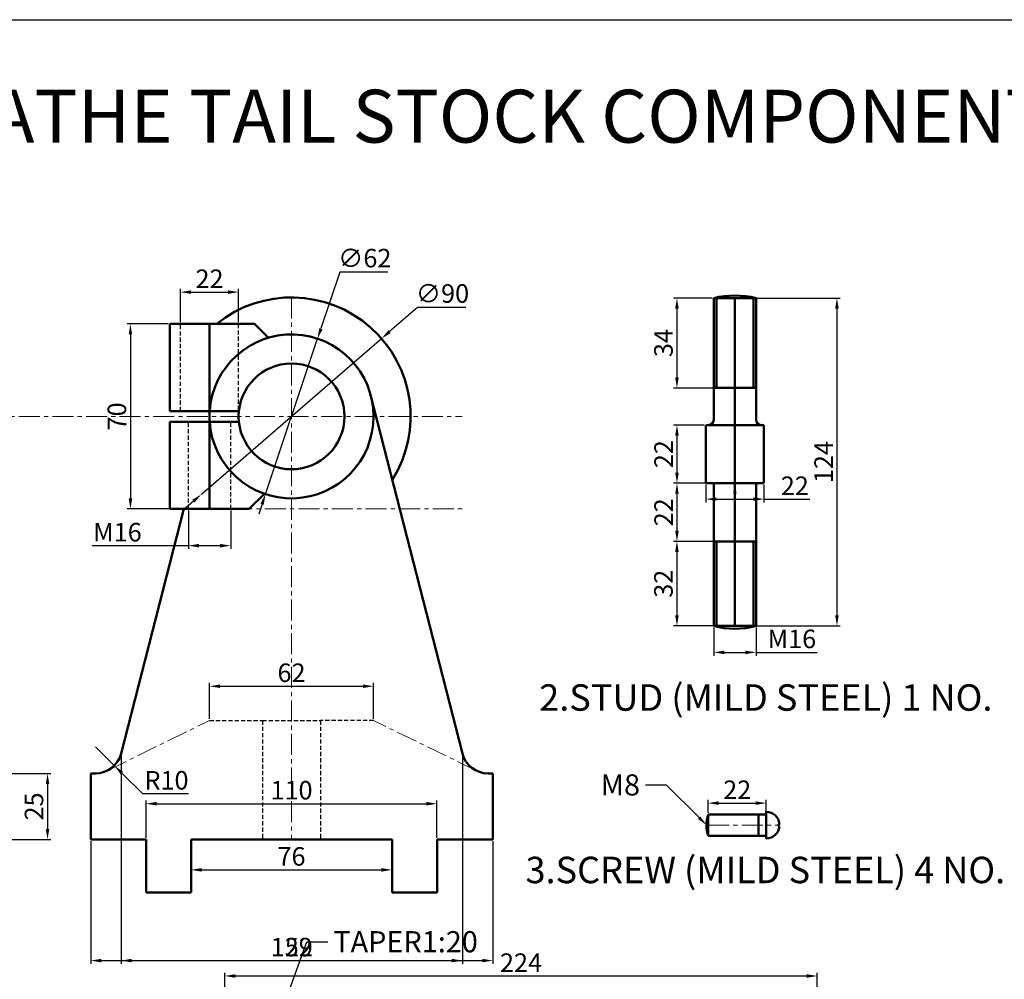
# Model space of a CAD drawing. Units: millimetres. Extents: x -66 to 1195, y -396 to 398.
# Tile 5 of 8: x 373 to 745, y 35 to 398. Entities that reach past the tile are written whole.
import ezdxf
from ezdxf import colors
from ezdxf.entities.mleader import LeaderData, LeaderLine
from ezdxf.math import Vec2, Vec3

# ---------------------------------------------------------------- set-up
doc = ezdxf.new("R2010")
doc.units = ezdxf.units.MM
doc.header["$LTSCALE"] = 0.5
doc.linetypes.add('CENTER', pattern=[50.8, 31.75, -6.35, 6.35, -6.35])
doc.linetypes.add('HIDDEN', pattern=[9.525, 6.35, -3.175])
for name, color, linetype, lineweight in [('M-CNTR', 1, 'CENTER', 18), ('M-DIMS', 2, 'Continuous', 25), ('M-HIDN', 3, 'HIDDEN', 25), ('M-OUTL', 7, 'Continuous', 50), ('M-TEXT', 7, 'Continuous', 25), ('M-TTLB', 7, 'Continuous', 25)]:
    doc.layers.add(name, color=color, linetype=linetype, lineweight=lineweight)
doc.styles.get("Standard").update_dxf_attribs({"font": 'arial.ttf'})
doc.dimstyles.new('ISO-25', dxfattribs={"dimtxt": 7, "dimasz": 4, "dimexe": 1.25, "dimexo": 0.625, "dimtad": 1, "dimtoh": 1, "dimtxsty": 'Standard', "dimcen": 2.5, "dimadec": 0, "dimazin": 0, "dimtfac": 1, "dimtmove": 0, "dimatfit": 3, "dimfxl": 1, "dimarcsym": 0})

# ---------------------------------------------------------------- blocks, each defined once
blk = doc.blocks.new('*D30')
at = {"layer": 'Defpoints', "color": 0, "ltscale": 0.5, "transparency": 16777216}
for p in [(185.07, 112.61), (185.07, 87.61), (383.19, 87.61)]:
    blk.add_point(p, dxfattribs=at)
at = {"layer": 'M-DIMS', "color": 0, "lineweight": -2, "ltscale": 0.5, "transparency": 16777216}
for p, q in [((185.69, 112.61), (384.44, 112.61)), ((383.19, 108.61), (383.19, 91.61)), ((185.69, 87.61), (384.44, 87.61))]:
    blk.add_line(p, q, dxfattribs=at)
at = {"layer": 'M-DIMS', "color": 0, "ltscale": 0.5, "transparency": 16777216}
for points in [[(382.52, 108.61), (383.85, 108.61), (383.19, 112.61)], [(382.52, 91.61), (383.85, 91.61), (383.19, 87.61)]]:
    blk.add_solid(points, dxfattribs=at)
at = {"layer": 'M-DIMS', "color": 0, "ltscale": 0.5, "transparency": 16777216, "insert": (378.99, 100.11), "char_height": 7, "attachment_point": 5, "rotation": 90}
blk.add_mtext('25', dxfattribs=at)
blk = doc.blocks.new('*D31')
at = {"layer": 'Defpoints', "color": 0, "ltscale": 0.5, "transparency": 16777216}
for p in [(506.43, 145.56), (444.43, 132.61), (506.43, 132.61)]:
    blk.add_point(p, dxfattribs=at)
at = {"layer": 'M-DIMS', "color": 0, "lineweight": -2, "ltscale": 0.5, "transparency": 16777216}
for p, q in [((444.43, 133.24), (444.43, 146.81)), ((448.43, 145.56), (502.43, 145.56)), ((506.43, 133.24), (506.43, 146.81))]:
    blk.add_line(p, q, dxfattribs=at)
at = {"layer": 'M-DIMS', "color": 0, "ltscale": 0.5, "transparency": 16777216}
for points in [[(448.43, 146.22), (448.43, 144.89), (444.43, 145.56)], [(502.43, 146.22), (502.43, 144.89), (506.43, 145.56)]]:
    blk.add_solid(points, dxfattribs=at)
at = {"layer": 'M-DIMS', "color": 0, "ltscale": 0.5, "transparency": 16777216, "insert": (475.43, 149.76), "char_height": 7, "attachment_point": 5}
blk.add_mtext('62', dxfattribs=at)
blk = doc.blocks.new('*D32')
at = {"layer": 'Defpoints', "color": 0, "ltscale": 0.5, "transparency": 16777216}
for p in [(530.43, 101.14), (420.43, 87.61), (530.43, 87.61)]:
    blk.add_point(p, dxfattribs=at)
at = {"layer": 'M-DIMS', "color": 0, "lineweight": -2, "ltscale": 0.5, "transparency": 16777216}
for p, q in [((420.43, 88.24), (420.43, 102.39)), ((424.43, 101.14), (526.43, 101.14)), ((530.43, 88.24), (530.43, 102.39))]:
    blk.add_line(p, q, dxfattribs=at)
at = {"layer": 'M-DIMS', "color": 0, "ltscale": 0.5, "transparency": 16777216}
for points in [[(424.43, 101.81), (424.43, 100.48), (420.43, 101.14)], [(526.43, 101.81), (526.43, 100.48), (530.43, 101.14)]]:
    blk.add_solid(points, dxfattribs=at)
at = {"layer": 'M-DIMS', "color": 0, "ltscale": 0.5, "transparency": 16777216, "insert": (475.43, 105.34), "char_height": 7, "attachment_point": 5}
blk.add_mtext('110', dxfattribs=at)
blk = doc.blocks.new('*D33')
at = {"layer": 'Defpoints', "color": 0, "ltscale": 0.5, "transparency": 16777216}
for p in [(437.43, 87.61), (513.43, 87.61), (513.43, 76.11)]:
    blk.add_point(p, dxfattribs=at)
at = {"layer": 'M-DIMS', "color": 0, "lineweight": -2, "ltscale": 0.5, "transparency": 16777216}
for p, q in [((437.43, 86.99), (437.43, 74.86)), ((513.43, 86.99), (513.43, 74.86)), ((441.43, 76.11), (509.43, 76.11))]:
    blk.add_line(p, q, dxfattribs=at)
at = {"layer": 'M-DIMS', "color": 0, "ltscale": 0.5, "transparency": 16777216}
for points in [[(441.43, 76.78), (441.43, 75.44), (437.43, 76.11)], [(509.43, 76.78), (509.43, 75.44), (513.43, 76.11)]]:
    blk.add_solid(points, dxfattribs=at)
at = {"layer": 'M-DIMS', "color": 0, "ltscale": 0.5, "transparency": 16777216, "insert": (475.43, 80.31), "char_height": 7, "attachment_point": 5}
blk.add_mtext('76', dxfattribs=at)
blk = doc.blocks.new('*D34')
at = {"layer": 'Defpoints', "color": 0, "ltscale": 0.5, "transparency": 16777216}
for p in [(429.43, 282.61), (414.53, 212.61), (429.43, 212.61)]:
    blk.add_point(p, dxfattribs=at)
at = {"layer": 'M-DIMS', "color": 0, "lineweight": -2, "ltscale": 0.5, "transparency": 16777216}
for p, q in [((428.81, 282.61), (413.28, 282.61)), ((414.53, 278.61), (414.53, 216.61)), ((428.81, 212.61), (413.28, 212.61))]:
    blk.add_line(p, q, dxfattribs=at)
at = {"layer": 'M-DIMS', "color": 0, "ltscale": 0.5, "transparency": 16777216}
for points in [[(413.87, 278.61), (415.2, 278.61), (414.53, 282.61)], [(413.87, 216.61), (415.2, 216.61), (414.53, 212.61)]]:
    blk.add_solid(points, dxfattribs=at)
at = {"layer": 'M-DIMS', "color": 0, "ltscale": 0.5, "transparency": 16777216, "insert": (410.33, 247.61), "char_height": 7, "attachment_point": 5, "rotation": 90}
blk.add_mtext('70', dxfattribs=at)
blk = doc.blocks.new('*D35')
at = {"layer": 'Defpoints', "color": 0, "ltscale": 0.5, "transparency": 16777216}
for p in [(455.43, 294.62), (433.43, 282.61), (455.43, 282.61)]:
    blk.add_point(p, dxfattribs=at)
at = {"layer": 'M-DIMS', "color": 0, "lineweight": -2, "ltscale": 0.5, "transparency": 16777216}
for p, q in [((433.43, 283.24), (433.43, 295.87)), ((437.43, 294.62), (451.43, 294.62)), ((455.43, 283.24), (455.43, 295.87))]:
    blk.add_line(p, q, dxfattribs=at)
at = {"layer": 'M-DIMS', "color": 0, "ltscale": 0.5, "transparency": 16777216}
for points in [[(437.43, 295.29), (437.43, 293.95), (433.43, 294.62)], [(451.43, 295.29), (451.43, 293.95), (455.43, 294.62)]]:
    blk.add_solid(points, dxfattribs=at)
at = {"layer": 'M-DIMS', "color": 0, "ltscale": 0.5, "transparency": 16777216, "insert": (444.43, 298.76), "char_height": 7, "attachment_point": 5}
blk.add_mtext('22', dxfattribs=at)
blk = doc.blocks.new('*D36')
at = {"layer": 'Defpoints', "color": 0, "ltscale": 0.5, "transparency": 16777216}
for p in [(436.43, 212.61), (452.43, 212.61), (452.43, 198.72)]:
    blk.add_point(p, dxfattribs=at)
at = {"layer": 'M-DIMS', "color": 0, "lineweight": -2, "ltscale": 0.5, "transparency": 16777216}
for p, q in [((436.43, 211.99), (436.43, 197.47)), ((452.43, 211.99), (452.43, 197.47)), ((436.43, 198.72), (400.07, 198.72)), ((448.43, 198.72), (440.43, 198.72))]:
    blk.add_line(p, q, dxfattribs=at)
at = {"layer": 'M-DIMS', "color": 0, "ltscale": 0.5, "transparency": 16777216}
for points in [[(440.43, 199.39), (440.43, 198.06), (436.43, 198.72)], [(448.43, 199.39), (448.43, 198.06), (452.43, 198.72)]]:
    blk.add_solid(points, dxfattribs=at)
at = {"layer": 'M-DIMS', "color": 0, "ltscale": 0.5, "transparency": 16777216, "insert": (409.62, 202.92), "char_height": 7, "attachment_point": 5}
blk.add_mtext('M16', dxfattribs=at)
blk = doc.blocks.new('*D37')
at = {"layer": 'Defpoints', "color": 0, "ltscale": 0.5, "transparency": 16777216}
for p in [(509.47, 277.04), (441.39, 218.18)]:
    blk.add_point(p, dxfattribs=at)
at = {"layer": 'M-DIMS', "color": 0, "lineweight": -2, "ltscale": 0.5, "transparency": 16777216}
for p, q in [((523.06, 288.79), (512.5, 279.66)), ((541.31, 288.79), (523.06, 288.79)), ((441.39, 218.18), (509.47, 277.04)), ((438.37, 215.56), (435.34, 212.95))]:
    blk.add_line(p, q, dxfattribs=at)
at = {"layer": 'M-DIMS', "color": 0, "ltscale": 0.5, "transparency": 16777216}
for points in [[(512.06, 280.16), (512.94, 279.15), (509.47, 277.04)], [(437.93, 216.07), (438.8, 215.06), (441.39, 218.18)]]:
    blk.add_solid(points, dxfattribs=at)
at = {"layer": 'M-DIMS', "color": 0, "ltscale": 0.5, "transparency": 16777216, "insert": (532.5, 293.19), "char_height": 7, "attachment_point": 5}
blk.add_mtext('∅90', dxfattribs=at)
blk = doc.blocks.new('*D38')
at = {"layer": 'Defpoints', "color": 0, "ltscale": 0.5, "transparency": 16777216}
for p in [(485.28, 277.01), (465.59, 218.22)]:
    blk.add_point(p, dxfattribs=at)
at = {"layer": 'M-DIMS', "color": 0, "lineweight": -2, "ltscale": 0.5, "transparency": 16777216}
for p, q in [((493.7, 302.17), (486.55, 280.8)), ((511.9, 302.17), (493.7, 302.17)), ((465.59, 218.22), (485.28, 277.01)), ((464.32, 214.42), (463.05, 210.63))]:
    blk.add_line(p, q, dxfattribs=at)
at = {"layer": 'M-DIMS', "color": 0, "ltscale": 0.5, "transparency": 16777216}
for points in [[(485.91, 281.01), (487.18, 280.59), (485.28, 277.01)], [(463.69, 214.63), (464.95, 214.21), (465.59, 218.22)]]:
    blk.add_solid(points, dxfattribs=at)
at = {"layer": 'M-DIMS', "color": 0, "ltscale": 0.5, "transparency": 16777216, "insert": (503.12, 306.57), "char_height": 7, "attachment_point": 5}
blk.add_mtext('∅62', dxfattribs=at)
blk = doc.blocks.new('*D39')
at = {"layer": 'Defpoints', "color": 0, "ltscale": 0.5, "transparency": 16777216}
for p in [(635.05, 292.35), (621.15, 258.35), (636.05, 258.35)]:
    blk.add_point(p, dxfattribs=at)
at = {"layer": 'M-DIMS', "color": 0, "lineweight": -2, "ltscale": 0.5, "transparency": 16777216}
for p, q in [((634.42, 292.35), (619.9, 292.35)), ((621.15, 288.35), (621.15, 262.35)), ((635.42, 258.35), (619.9, 258.35))]:
    blk.add_line(p, q, dxfattribs=at)
at = {"layer": 'M-DIMS', "color": 0, "ltscale": 0.5, "transparency": 16777216}
for points in [[(620.48, 288.35), (621.81, 288.35), (621.15, 292.35)], [(620.48, 262.35), (621.81, 262.35), (621.15, 258.35)]]:
    blk.add_solid(points, dxfattribs=at)
at = {"layer": 'M-DIMS', "color": 0, "ltscale": 0.5, "transparency": 16777216, "insert": (616.95, 275.35), "char_height": 7, "attachment_point": 5, "rotation": 90}
blk.add_mtext('34', dxfattribs=at)
blk = doc.blocks.new('*D40')
at = {"layer": 'Defpoints', "color": 0, "ltscale": 0.5, "transparency": 16777216}
for p in [(632.05, 222.35), (654.05, 222.35), (654.05, 216.33)]:
    blk.add_point(p, dxfattribs=at)
at = {"layer": 'M-DIMS', "color": 0, "lineweight": -2, "ltscale": 0.5, "transparency": 16777216}
for p, q in [((632.05, 221.73), (632.05, 215.08)), ((654.05, 221.73), (654.05, 215.08)), ((636.05, 216.33), (650.05, 216.33)), ((654.05, 216.33), (671.37, 216.33))]:
    blk.add_line(p, q, dxfattribs=at)
at = {"layer": 'M-DIMS', "color": 0, "ltscale": 0.5, "transparency": 16777216}
for points in [[(636.05, 216.99), (636.05, 215.66), (632.05, 216.33)], [(650.05, 216.99), (650.05, 215.66), (654.05, 216.33)]]:
    blk.add_solid(points, dxfattribs=at)
at = {"layer": 'M-DIMS', "color": 0, "ltscale": 0.5, "transparency": 16777216, "insert": (665.71, 220.47), "char_height": 7, "attachment_point": 5}
blk.add_mtext('22', dxfattribs=at)
blk = doc.blocks.new('*D41')
at = {"layer": 'Defpoints', "color": 0, "ltscale": 0.5, "transparency": 16777216}
for p in [(632.05, 244.35), (621.15, 222.35), (632.05, 222.35)]:
    blk.add_point(p, dxfattribs=at)
at = {"layer": 'M-DIMS', "color": 0, "lineweight": -2, "ltscale": 0.5, "transparency": 16777216}
for p, q in [((631.42, 244.35), (619.9, 244.35)), ((621.15, 240.35), (621.15, 226.35)), ((631.42, 222.35), (619.9, 222.35))]:
    blk.add_line(p, q, dxfattribs=at)
at = {"layer": 'M-DIMS', "color": 0, "ltscale": 0.5, "transparency": 16777216}
for points in [[(620.48, 240.35), (621.81, 240.35), (621.15, 244.35)], [(620.48, 226.35), (621.81, 226.35), (621.15, 222.35)]]:
    blk.add_solid(points, dxfattribs=at)
at = {"layer": 'M-DIMS', "color": 0, "ltscale": 0.5, "transparency": 16777216, "insert": (617.01, 233.35), "char_height": 7, "attachment_point": 5, "rotation": 90}
blk.add_mtext('22', dxfattribs=at)
blk = doc.blocks.new('*D42')
at = {"layer": 'Defpoints', "color": 0, "ltscale": 0.5, "transparency": 16777216}
for p in [(643.05, 222.35), (621.15, 200.35), (643.05, 200.35)]:
    blk.add_point(p, dxfattribs=at)
at = {"layer": 'M-DIMS', "color": 0, "lineweight": -2, "ltscale": 0.5, "transparency": 16777216}
for p, q in [((642.42, 222.35), (619.9, 222.35)), ((621.15, 218.35), (621.15, 204.35)), ((642.42, 200.35), (619.9, 200.35))]:
    blk.add_line(p, q, dxfattribs=at)
at = {"layer": 'M-DIMS', "color": 0, "ltscale": 0.5, "transparency": 16777216}
for points in [[(620.48, 218.35), (621.81, 218.35), (621.15, 222.35)], [(620.48, 204.35), (621.81, 204.35), (621.15, 200.35)]]:
    blk.add_solid(points, dxfattribs=at)
at = {"layer": 'M-DIMS', "color": 0, "ltscale": 0.5, "transparency": 16777216, "insert": (617.01, 211.35), "char_height": 7, "attachment_point": 5, "rotation": 90}
blk.add_mtext('22', dxfattribs=at)
blk = doc.blocks.new('*D43')
at = {"layer": 'Defpoints', "color": 0, "ltscale": 0.5, "transparency": 16777216}
for p in [(643.05, 200.35), (621.15, 168.35), (643.05, 168.35)]:
    blk.add_point(p, dxfattribs=at)
at = {"layer": 'M-DIMS', "color": 0, "lineweight": -2, "ltscale": 0.5, "transparency": 16777216}
for p, q in [((642.42, 200.35), (619.9, 200.35)), ((621.15, 196.35), (621.15, 172.35)), ((642.42, 168.35), (619.9, 168.35))]:
    blk.add_line(p, q, dxfattribs=at)
at = {"layer": 'M-DIMS', "color": 0, "ltscale": 0.5, "transparency": 16777216}
for points in [[(620.48, 196.35), (621.81, 196.35), (621.15, 200.35)], [(620.48, 172.35), (621.81, 172.35), (621.15, 168.35)]]:
    blk.add_solid(points, dxfattribs=at)
at = {"layer": 'M-DIMS', "color": 0, "ltscale": 0.5, "transparency": 16777216, "insert": (616.95, 184.35), "char_height": 7, "attachment_point": 5, "rotation": 90}
blk.add_mtext('32', dxfattribs=at)
blk = doc.blocks.new('*D44')
at = {"layer": 'Defpoints', "color": 0, "ltscale": 0.5, "transparency": 16777216}
for p in [(635.05, 168.35), (651.05, 168.35), (651.05, 158.37)]:
    blk.add_point(p, dxfattribs=at)
at = {"layer": 'M-DIMS', "color": 0, "lineweight": -2, "ltscale": 0.5, "transparency": 16777216}
for p, q in [((635.05, 167.73), (635.05, 157.12)), ((651.05, 167.73), (651.05, 157.12)), ((639.05, 158.37), (647.05, 158.37)), ((651.05, 158.37), (674.15, 158.37))]:
    blk.add_line(p, q, dxfattribs=at)
at = {"layer": 'M-DIMS', "color": 0, "ltscale": 0.5, "transparency": 16777216}
for points in [[(639.05, 159.04), (639.05, 157.7), (635.05, 158.37)], [(647.05, 159.04), (647.05, 157.7), (651.05, 158.37)]]:
    blk.add_solid(points, dxfattribs=at)
at = {"layer": 'M-DIMS', "color": 0, "ltscale": 0.5, "transparency": 16777216, "insert": (664.6, 162.57), "char_height": 7, "attachment_point": 5}
blk.add_mtext('M16', dxfattribs=at)
blk = doc.blocks.new('*D45')
at = {"layer": 'Defpoints', "color": 0, "ltscale": 0.5, "transparency": 16777216}
for p in [(643.05, 292.35), (643.05, 168.35), (681.63, 168.35)]:
    blk.add_point(p, dxfattribs=at)
at = {"layer": 'M-DIMS', "color": 0, "lineweight": -2, "ltscale": 0.5, "transparency": 16777216}
for p, q in [((643.67, 292.35), (682.88, 292.35)), ((681.63, 288.35), (681.63, 172.35)), ((643.67, 168.35), (682.88, 168.35))]:
    blk.add_line(p, q, dxfattribs=at)
at = {"layer": 'M-DIMS', "color": 0, "ltscale": 0.5, "transparency": 16777216}
for points in [[(680.97, 288.35), (682.3, 288.35), (681.63, 292.35)], [(680.97, 172.35), (682.3, 172.35), (681.63, 168.35)]]:
    blk.add_solid(points, dxfattribs=at)
at = {"layer": 'M-DIMS', "color": 0, "ltscale": 0.5, "transparency": 16777216, "insert": (677.49, 230.35), "char_height": 7, "attachment_point": 5, "rotation": 90}
blk.add_mtext('124', dxfattribs=at)
blk = doc.blocks.new('*D46')
at = {"layer": 'Defpoints', "color": 0, "ltscale": 0.5, "transparency": 16777216}
for p in [(654.93, 101.37), (632.93, 97.04), (654.93, 97.54)]:
    blk.add_point(p, dxfattribs=at)
at = {"layer": 'M-DIMS', "color": 0, "lineweight": -2, "ltscale": 0.5, "transparency": 16777216}
for p, q in [((632.93, 97.67), (632.93, 102.62)), ((636.93, 101.37), (650.93, 101.37)), ((654.93, 98.17), (654.93, 102.62))]:
    blk.add_line(p, q, dxfattribs=at)
at = {"layer": 'M-DIMS', "color": 0, "ltscale": 0.5, "transparency": 16777216}
for points in [[(636.93, 102.04), (636.93, 100.7), (632.93, 101.37)], [(650.93, 102.04), (650.93, 100.7), (654.93, 101.37)]]:
    blk.add_solid(points, dxfattribs=at)
at = {"layer": 'M-DIMS', "color": 0, "ltscale": 0.5, "transparency": 16777216, "insert": (643.93, 105.51), "char_height": 7, "attachment_point": 5}
blk.add_mtext('22', dxfattribs=at)
blk = doc.blocks.new('*D50')
at = {"layer": 'Defpoints', "color": 0, "ltscale": 0.5, "transparency": 16777216}
for p in [(674.2, 35.99), (450.2, 28.9), (674.2, 28.9)]:
    blk.add_point(p, dxfattribs=at)
at = {"layer": 'M-DIMS', "color": 0, "lineweight": -2, "ltscale": 0.5, "transparency": 16777216}
for p, q in [((450.2, 29.53), (450.2, 37.24)), ((674.2, 29.53), (674.2, 37.24)), ((454.2, 35.99), (670.2, 35.99))]:
    blk.add_line(p, q, dxfattribs=at)
at = {"layer": 'M-DIMS', "color": 0, "ltscale": 0.5, "transparency": 16777216}
for points in [[(454.2, 36.65), (454.2, 35.32), (450.2, 35.99)], [(670.2, 36.65), (670.2, 35.32), (674.2, 35.99)]]:
    blk.add_solid(points, dxfattribs=at)
at = {"layer": 'M-DIMS', "color": 0, "ltscale": 0.5, "transparency": 16777216, "insert": (562.2, 40.13), "char_height": 7, "attachment_point": 5}
blk.add_mtext('224', dxfattribs=at)
blk = doc.blocks.new('*D103')
at = {"layer": 'Defpoints', "color": 0, "ltscale": 0.5, "transparency": 16777216}
for p in [(399.53, 87.61), (551.53, 87.61), (551.53, 41.81)]:
    blk.add_point(p, dxfattribs=at)
at = {"layer": 'M-DIMS', "color": 0, "lineweight": -2, "ltscale": 0.5, "transparency": 16777216}
for p, q in [((399.53, 86.99), (399.53, 40.56)), ((551.53, 86.99), (551.53, 40.56)), ((403.53, 41.81), (547.53, 41.81))]:
    blk.add_line(p, q, dxfattribs=at)
at = {"layer": 'M-DIMS', "color": 0, "ltscale": 0.5, "transparency": 16777216}
for points in [[(403.53, 42.48), (403.53, 41.14), (399.53, 41.81)], [(547.53, 42.48), (547.53, 41.14), (551.53, 41.81)]]:
    blk.add_solid(points, dxfattribs=at)
at = {"layer": 'M-DIMS', "color": 0, "ltscale": 0.5, "transparency": 16777216, "insert": (475.53, 46.01), "char_height": 7, "attachment_point": 5}
blk.add_mtext('152', dxfattribs=at)
blk = doc.blocks.new('*D104')
at = {"layer": 'Defpoints', "color": 0, "ltscale": 0.5, "transparency": 16777216}
for p in [(411.03, 120.13), (540.03, 120.13), (540.03, 41.81)]:
    blk.add_point(p, dxfattribs=at)
at = {"layer": 'M-DIMS', "color": 0, "lineweight": -2, "ltscale": 0.5, "transparency": 16777216}
for p, q in [((411.03, 119.51), (411.03, 40.56)), ((540.03, 119.51), (540.03, 40.56)), ((415.03, 41.81), (536.03, 41.81))]:
    blk.add_line(p, q, dxfattribs=at)
at = {"layer": 'M-DIMS', "color": 0, "ltscale": 0.5, "transparency": 16777216}
for points in [[(415.03, 42.48), (415.03, 41.14), (411.03, 41.81)], [(536.03, 42.48), (536.03, 41.14), (540.03, 41.81)]]:
    blk.add_solid(points, dxfattribs=at)
at = {"layer": 'M-DIMS', "color": 0, "ltscale": 0.5, "transparency": 16777216, "insert": (475.53, 46.01), "char_height": 7, "attachment_point": 5}
blk.add_mtext('129', dxfattribs=at)
blk = doc.blocks.new('*D118')
at = {"layer": 'Defpoints', "color": 0, "ltscale": 0.5, "transparency": 16777216}
for p in [(401.34, 122.61), (408.44, 115.56)]:
    blk.add_point(p, dxfattribs=at)
at = {"layer": 'M-DIMS', "color": 0, "lineweight": -2, "ltscale": 0.5, "transparency": 16777216}
for p, q in [((401.34, 122.61), (408.44, 115.56)), ((419.18, 104.89), (411.27, 112.74)), ((436.51, 104.89), (419.18, 104.89))]:
    blk.add_line(p, q, dxfattribs=at)
at = {"layer": 'M-DIMS', "color": 0, "ltscale": 0.5, "transparency": 16777216}
blk.add_solid([(411.74, 113.22), (410.8, 112.27), (408.44, 115.56)], dxfattribs=at)
at = {"layer": 'M-DIMS', "color": 0, "ltscale": 0.5, "transparency": 16777216, "insert": (428.16, 109.09), "char_height": 7, "attachment_point": 5}
blk.add_mtext('R10', dxfattribs=at)

msp = doc.modelspace()

# ---------------------------------------------------------------- linework, layer by layer
at = {"layer": 'M-CNTR', "ltscale": 0.5}
for p, q in [((475.4327, 292.6106), (475.4327, 87.6106)), ((346.9367, 247.6106), (539.9794, 247.6106)), ((414.5332, 212.6106), (539.9794, 212.6106)), ((405.7453, 113.6326), (444.4327, 132.6106)), ((545.3342, 113.6238), (506.4327, 132.6106)), ((632.9262, 93.0426), (659.3995, 93.0426))]:
    msp.add_line(p, q, dxfattribs=at)
at = {"layer": 'M-HIDN', "ltscale": 0.5}
for p, q in [((433.4327, 249.6106), (433.4327, 282.6106)), ((455.4327, 247.6106), (455.4327, 282.6106)), ((436.4327, 212.6106), (436.4327, 245.6106)), ((452.4327, 212.6106), (452.4327, 245.6106)), ((444.4327, 132.6106), (464.4327, 132.6106)), ((464.4327, 132.6106), (486.4327, 132.6106)), ((464.4327, 132.6106), (464.4327, 87.6106)), ((486.4327, 132.6106), (486.4327, 87.6106)), ((506.4327, 132.6106), (486.4327, 132.6106))]:
    msp.add_line(p, q, dxfattribs=at)
at = {"layer": 'M-OUTL', "ltscale": 0.5}
for p, q in [((635.0478, 292.3534), (651.0478, 292.3534)), ((635.0478, 246.3534), (635.0478, 292.3534)), ((636.0478, 258.3534), (636.0478, 292.3534)), ((643.0478, 292.3534), (643.0478, 168.3534)), ((650.0478, 292.3534), (650.0478, 258.3534)), ((651.0478, 292.3534), (651.0478, 246.3534)), ((429.4327, 249.6106), (429.4327, 282.6106)), ((429.4327, 282.6106), (461.4327, 282.6106)), ((444.4327, 249.6106), (444.4327, 282.6106)), ((461.4327, 282.6106), (466.6908, 277.3525)), ((651.0478, 258.3534), (635.0478, 258.3534)), ((643.0478, 258.3534), (643.0478, 242.3534)), ((505.4661, 255.2915), (540.0322, 120.1329)), ((429.4327, 249.6106), (455.533, 249.6106)), ((444.4327, 212.6106), (444.4327, 249.6106)), ((429.4327, 212.6106), (429.4327, 245.6106)), ((429.4327, 245.6106), (455.533, 245.6106)), ((632.0478, 244.3534), (632.0478, 222.3534)), ((633.0478, 244.3534), (632.0478, 244.3534)), ((654.0478, 244.3534), (633.0478, 244.3534)), ((654.0478, 244.3534), (654.0478, 222.3534)), ((632.0478, 222.3534), (654.0478, 222.3534)), ((635.0478, 222.3534), (635.0478, 168.3534)), ((643.0478, 222.3534), (643.0478, 200.3534)), ((643.0478, 222.3534), (643.0478, 200.3534)), ((651.0478, 222.3534), (651.0478, 168.3534)), ((459.4327, 212.6106), (465.178, 218.3558)), ((434.6801, 212.6106), (411.0294, 120.1329)), ((429.4327, 212.6106), (459.4327, 212.6106)), ((635.0478, 200.3534), (651.0478, 200.3534)), ((636.0478, 200.3534), (636.0478, 168.3534)), ((650.0478, 200.3534), (650.0478, 168.3534)), ((635.0478, 168.3534), (651.0478, 168.3534)), ((399.5308, 112.6106), (401.3412, 112.6106)), ((399.5308, 112.6106), (399.5308, 87.6106)), ((549.7204, 112.6106), (551.5308, 112.6106)), ((551.5308, 112.6106), (551.5308, 87.6106)), ((632.9262, 97.0426), (654.9262, 97.0426)), ((632.9262, 89.0426), (632.9262, 97.0426)), ((651.9262, 97.0426), (651.9262, 89.0426)), ((654.9262, 97.0426), (654.9262, 98.0426)), ((654.9262, 97.0426), (654.9262, 89.0426)), ((659.901, 93.5441), (659.3995, 93.0426)), ((659.901, 92.541), (659.3995, 93.0426)), ((399.5308, 87.6106), (420.4327, 87.6106)), ((420.4327, 87.6106), (420.4327, 67.6106)), ((437.4327, 87.6106), (437.4327, 67.6106)), ((437.4327, 87.6106), (513.4327, 87.6106)), ((513.4327, 87.6106), (513.4327, 67.6106)), ((530.4327, 87.6106), (530.4327, 67.6106)), ((530.4327, 87.6106), (551.5308, 87.6106)), ((654.9262, 89.0426), (632.9262, 89.0426)), ((654.9262, 89.0426), (654.9262, 88.0426)), ((420.4327, 67.6106), (437.4327, 67.6106)), ((513.4327, 67.6106), (530.4327, 67.6106))]:
    msp.add_line(p, q, dxfattribs=at)
msp.add_circle((475.4327, 247.6106), 20, dxfattribs=at)
for centre, radius, start, end in [((475.4327, 247.6106), 45, 327.887824, 128.942441), ((643.0478, 259.7431), 33.5772, 76.21633, 103.78367), ((475.4327, 247.6106), 31, 183.699071, 176.300929), ((633.0478, 246.3534), 2, 270, 0), ((653.0478, 246.3534), 2, 180, 270), ((643.0478, 198.7001), 31.3835, 255.231697, 284.768303), ((401.3412, 122.6106), 10, 270, 345.654395), ((549.7204, 122.6106), 10, 194.345605, 270), ((646.2508, 93.0426), 13.9121, 163.290472, 196.709528), ((654.9262, 93.0426), 5, 5.75663, 90), ((654.9262, 93.0426), 5, 270, 354.24337)]:
    msp.add_arc(centre, radius, start, end, dxfattribs=at)
at = {"layer": 'M-TTLB', "ltscale": 0.5}
msp.add_lwpolyline([(-66.4176, 397.641), (1195.0519, 397.641), (1195.0519, -395.6964), (-66.4176, -395.6964)], close=True, dxfattribs=at)

# ---------------------------------------------------------------- texts
at = {"layer": 'M-TEXT', "ltscale": 0.5, "attachment_point": 1}
for s, width, insert, char_height in [('LATHE TAIL STOCK COMPONENTS ', 485.790741, (346.8576, 371.1482), 20), ('\\pxqc;2.STUD (MILD STEEL) 1 NO.', 191.333714, (559.0807, 146.3007), 10), ('\\pxqc;3.SCREW (MILD STEEL) 4 NO.', 203.992441, (552.5644, 81.0812), 10)]:
    msp.add_mtext_dynamic_manual_height_columns(s, width=width, gutter_width=12.5, heights=[0], dxfattribs=dict(at, insert=insert, char_height=char_height))

# ---------------------------------------------------------------- dimensions: what is measured, and where the dimension line sits
at = {"layer": 'M-DIMS', "ltscale": 0.5}
for p1, p2, picture, middle in [((465.5888, 218.215), (485.2766, 277.0061), '*D38', (503.1153, 302.1731)), ((441.3921, 218.1787), (509.4733, 277.0425), '*D37', (532.4958, 288.7907))]:
    dim = msp.add_diameter_dim_2p(p1=p1, p2=p2, dimstyle='ISO-25', override={"dimclrd": 0, "dimclre": 0, "dimclrt": 0}, dxfattribs=at)
    dim.commit()
    dim.dimension.update_dxf_attribs({"geometry": picture, "text_midpoint": middle, "dimtype": 163})
for base, p1, p2, override, picture, middle in [((455.4327, 294.621), (433.4327, 282.6106), (455.4327, 282.6106), {"dimclrd": 0, "dimclre": 0, "dimclrt": 0}, '*D35', (444.4327, 298.7604)), ((506.4327, 145.5566), (444.4327, 132.6106), (506.4327, 132.6106), {"dimclrd": 0, "dimclre": 0, "dimclrt": 0}, '*D31', (475.4327, 149.7556)), ((540.0322, 41.8106), (411.0294, 120.1329), (540.0322, 120.1329), {"dimdec": 0, "dimlfac": 1, "dimrnd": 0, "dimzin": 0, "dimdsep": 46, "dimlunit": 2}, '*D104', (475.5308, 46.0096)), ((530.4327, 101.1427), (420.4327, 87.6106), (530.4327, 87.6106), {"dimclrd": 0, "dimclre": 0, "dimclrt": 0}, '*D32', (475.4327, 105.3417)), ((654.9262, 101.3698), (632.9262, 97.0426), (654.9262, 97.5426), {"dimclrd": 0, "dimclre": 0, "dimclrt": 0}, '*D46', (643.9262, 105.5091)), ((551.5308, 41.8106), (399.5308, 87.6106), (551.5308, 87.6106), {"dimdec": 0, "dimlfac": 1, "dimrnd": 0, "dimzin": 0, "dimdsep": 46, "dimlunit": 2}, '*D103', (475.5308, 46.0096)), ((513.4327, 76.1101), (437.4327, 87.6106), (513.4327, 87.6106), {"dimclrd": 0, "dimclre": 0, "dimclrt": 0}, '*D33', (475.4327, 80.3091)), ((674.1953, 35.9864), (450.1953, 28.9037), (674.1953, 28.9037), {"dimclrd": 0, "dimclre": 0, "dimclrt": 0}, '*D50', (562.1953, 40.1258))]:
    dim = msp.add_linear_dim(base=base, p1=p1, p2=p2, dimstyle='ISO-25', override=override, dxfattribs=at)
    dim.commit()
    dim.dimension.update_dxf_attribs({"geometry": picture, "text_midpoint": middle})
for base, p1, p2, picture, middle in [((621.1467, 258.3534), (635.0478, 292.3534), (636.0478, 258.3534), '*D39', (616.9453, 275.3534)), ((681.6328, 168.3534), (643.0478, 292.3534), (643.0478, 168.3534), '*D45', (677.4935, 230.3534)), ((414.5332, 212.6106), (429.4327, 282.6106), (429.4327, 212.6106), '*D34', (410.3342, 247.6106)), ((621.1467, 222.3534), (632.0478, 244.3534), (632.0478, 222.3534), '*D41', (617.0073, 233.3534)), ((621.1467, 200.3534), (643.0478, 222.3534), (643.0478, 200.3534), '*D42', (617.0073, 211.3534)), ((621.1467, 168.3534), (643.0478, 200.3534), (643.0478, 168.3534), '*D43', (616.9453, 184.3534)), ((383.1852, 87.6106), (185.0679, 112.6106), (185.0679, 87.6106), '*D30', (378.9862, 100.1106))]:
    dim = msp.add_linear_dim(base=base, p1=p1, p2=p2, angle=90, dimstyle='ISO-25', override={"dimclrd": 0, "dimclre": 0, "dimclrt": 0}, dxfattribs=at)
    dim.commit()
    dim.dimension.update_dxf_attribs({"geometry": picture, "text_midpoint": middle})
dim = msp.add_linear_dim(base=(654.0478, 216.3266), p1=(632.0478, 222.3534), p2=(654.0478, 222.3534), dimstyle='ISO-25', override={"dimclrd": 0, "dimclre": 0, "dimclrt": 0}, dxfattribs=at)
dim.commit()
dim.dimension.update_dxf_attribs({"geometry": '*D40', "text_midpoint": (665.7112, 216.3266), "dimtype": 160})
dim = msp.add_linear_dim(base=(452.4327, 198.7221), p1=(436.4327, 212.6106), p2=(452.4327, 212.6106), text='M<>', dimstyle='ISO-25', override={"dimclrd": 0, "dimclre": 0, "dimclrt": 0}, dxfattribs=at)
dim.commit()
dim.dimension.update_dxf_attribs({"geometry": '*D36', "text_midpoint": (409.6222, 198.7221), "dimtype": 160})
dim = msp.add_linear_dim(base=(651.0478, 158.3685), p1=(635.0478, 168.3534), p2=(651.0478, 168.3534), text='M<>', dimstyle='ISO-25', override={"dimclrd": 0, "dimclre": 0, "dimclrt": 0}, dxfattribs=at)
dim.commit()
dim.dimension.update_dxf_attribs({"geometry": '*D44', "text_midpoint": (664.5971, 162.5675)})
dim = msp.add_radius_dim(center=(401.3412, 122.6106), mpoint=(408.4361, 115.5634), dimstyle='ISO-25', override={"dimdec": 0, "dimlfac": 1, "dimrnd": 0, "dimzin": 0, "dimdsep": 46, "dimlunit": 2}, dxfattribs=at)
dim.commit()
dim.dimension.update_dxf_attribs({"geometry": '*D118', "text_midpoint": (428.1598, 109.0874)})

# ---------------------------------------------------------------- leaders
at = {"layer": 'M-TEXT', "ltscale": 0.5}
ml = msp.add_multileader_mtext('Standard', dxfattribs=at)
ml.set_content('', color=256)
ml.set_leader_properties()
ml.build(insert=Vec2(0, 0))
ctx = ml.context
ctx.base_point, ctx.plane_origin = Vec3(651.0478, 200.3534), Vec3(643.0478, 222.3534)
notes = []
notes.append((ctx, [(0, (1, 1, 0), (643.0478, 200.3534), (1, 0), 8, [(0, [(643.0478, 222.3534)], 0, [])])]))
ctx.mtext.insert, ctx.mtext.flow_direction = Vec3(653.0478, 202.3534), 5
ml = msp.add_multileader_mtext('Standard', dxfattribs=at)
ml.set_content('M8', color=256)
ml.set_leader_properties()
ml.build(insert=Vec2(0, 0))
ctx = ml.context
ctx.base_point, ctx.char_height, ctx.plane_origin = Vec3(590.9961, 108.1806), 8, Vec3(632.3388, 93.0426)
ctx.text_align_type = 2
notes.append((ctx, [(0, (1, 1, 0), (617.2007, 108.1806), (-1, 0), 8, [(0, [(632.3388, 93.0426)], 0, [])])]))
ctx.mtext.insert, ctx.mtext.alignment, ctx.mtext.flow_direction = Vec3(607.2007, 112.2488), 3, 5
ml = msp.add_multileader_mtext('Standard', dxfattribs=at)
ml.set_content('TAPER1:20', color=256)
ml.set_leader_properties()
ml.build(insert=Vec2(0, 0))
ctx = ml.context
ctx.base_point, ctx.char_height, ctx.plane_origin = Vec3(489.22, 48.8808), 8, Vec3(470.1953, 18.4037)
notes.append((ctx, [(0, (1, 1, 0), (481.22, 48.8808), (1, 0), 8, [(0, [(470.1953, 18.4037)], 0, [])])]))
ctx.mtext.insert, ctx.mtext.flow_direction = Vec3(491.22, 52.949), 5
for ctx, leaders in notes:
    for number, flags, end, landing, length, lines in leaders:
        leader = LeaderData()
        leader.index, (leader.has_last_leader_line, leader.has_dogleg_vector, leader.attachment_direction) = number, flags
        leader.last_leader_point, leader.dogleg_vector, leader.dogleg_length = Vec3(end), Vec3(landing), length
        for number, points, colour, breaks in lines:
            line = LeaderLine()
            line.index, line.vertices, line.color, line.breaks = number, Vec3.list(points), colors.encode_raw_color(colour), breaks
            leader.lines.append(line)
        ctx.leaders.append(leader)

doc.saveas('drawing.dxf')
